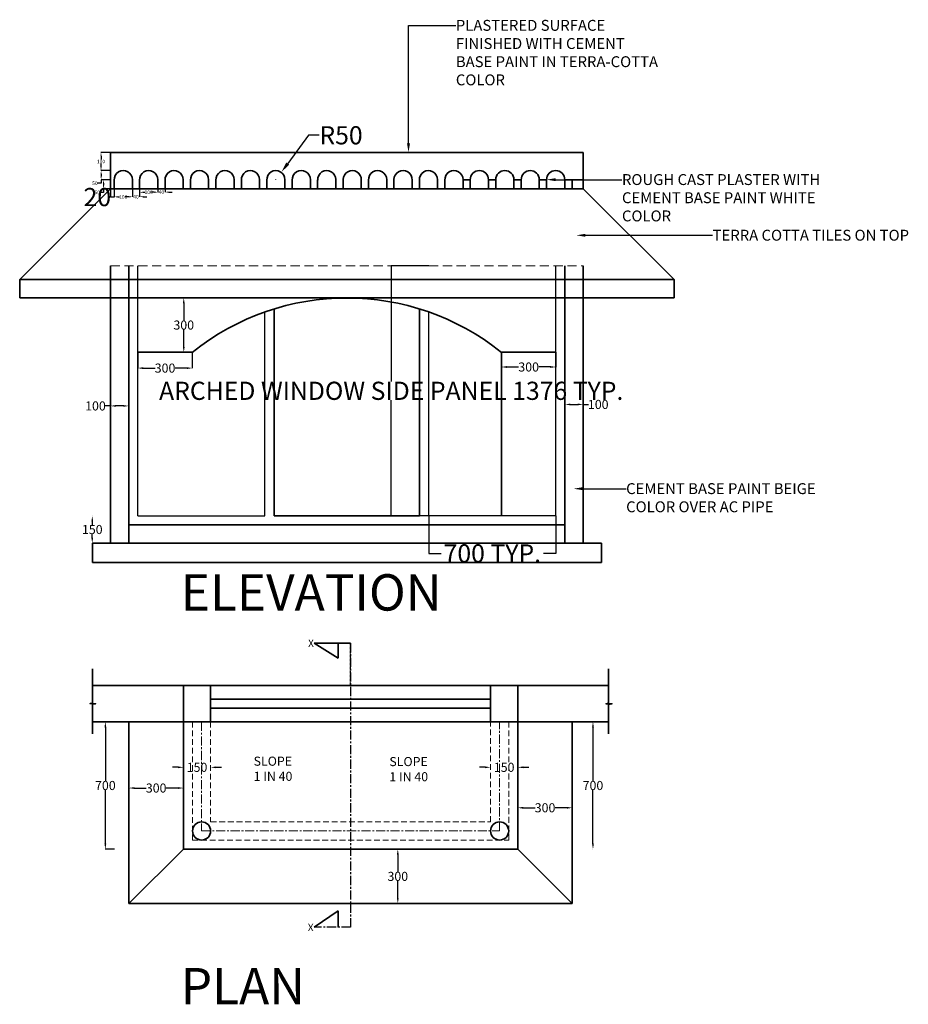
# Model space of a CAD drawing. Units: millimetres. Extents: x 12559 to 31551, y 33148 to 41181.
# Tile 1 of 3: x 12559 to 17450, y 35764 to 41181. Entities that reach past the tile are written whole.
import ezdxf
from ezdxf import colors
from ezdxf.entities.mleader import LeaderData, LeaderLine
from ezdxf.math import Vec2, Vec3

# ---------------------------------------------------------------- set-up
doc = ezdxf.new("R2010")
doc.units = ezdxf.units.MM
doc.header["$MEASUREMENT"] = 0
doc.linetypes.add('CENTER', pattern=[2, 1.25, -0.25, 0.25, -0.25])
doc.linetypes.add('HIDDEN', pattern=[9.525, 6.35, -3.175])
for name, color, linetype, lineweight in [('A-ANNO-DIMS', 2, 'Continuous', 18), ('A-ANNO-SYMB', 2, 'CENTER', 25), ('A-ANNO-TEXT', 3, 'Continuous', 25), ('A-DETL', 7, 'Continuous', 35), ('A-DETL-CNTR', 1, 'CENTER', 18), ('A-DETL-HIDN', 8, 'HIDDEN', 18), ('A-ELEV', 7, 'Continuous', 35), ('A-ELEV-HIDN', 8, 'HIDDEN', 18), ('A-GLAZ', 4, 'Continuous', 25)]:
    doc.layers.add(name, color=color, linetype=linetype, lineweight=lineweight)
doc.styles.get("Standard").update_dxf_attribs({"font": 'arial.ttf'})
doc.dimstyles.get("Standard").update_dxf_attribs({"dimtxt": 100, "dimasz": 0.18, "dimexe": 0.18, "dimexo": 0.0625, "dimgap": 0.09, "dimtad": 0, "dimtih": 1, "dimtoh": 1, "dimdec": 0, "dimzin": 0, "dimdsep": 46, "dimtxsty": 'Standard', "dimcen": 0.09, "dimadec": 0, "dimazin": 0, "dimtfac": 1, "dimtdec": 0, "dimtofl": 0, "dimtmove": 0, "dimatfit": 3, "dimfxl": 1, "dimtolj": 1, "dimtzin": 0, "dimarcsym": 0})

# ---------------------------------------------------------------- blocks, each defined once
blk = doc.blocks.new('*D2')
at = {"layer": 'A-ANNO-DIMS', "color": 0, "lineweight": -2, "transparency": 16777216}
for p, q in [((13430.3, 37067.5), (13400.3, 37067.5)), ((13460.3, 37067.6), (13460.3, 37067.7)), ((13610.3, 37067.6), (13610.3, 37067.7)), ((13640.3, 37067.5), (13670.3, 37067.5))]:
    blk.add_line(p, q, dxfattribs=at)
at = {"layer": 'A-ANNO-DIMS', "color": 0, "transparency": 16777216}
for points in [[(13430.3, 37072.5), (13430.3, 37062.5), (13460.3, 37067.5)], [(13640.3, 37072.5), (13640.3, 37062.5), (13610.3, 37067.5)]]:
    blk.add_solid(points, dxfattribs=at)
at = {"layer": 'DEFPOINTS', "color": 0, "transparency": 16777216}
for p in [(13460.3, 37067.5), (13610.3, 37067.5), (13610.3, 37067.5)]:
    blk.add_point(p, dxfattribs=at)
at = {"layer": 'A-ANNO-DIMS', "color": 0, "transparency": 16777216, "insert": (13535.3, 37067.5), "char_height": 50, "attachment_point": 5}
blk.add_mtext('\\A1;150', dxfattribs=at)
blk = doc.blocks.new('*D3')
at = {"layer": 'A-ANNO-DIMS', "color": 0, "lineweight": -2, "transparency": 16777216}
for p, q in [((15120.7, 37067.5), (15090.7, 37067.5)), ((15150.7, 37067.6), (15150.7, 37067.7)), ((15300.7, 37067.6), (15300.7, 37067.7)), ((15330.7, 37067.5), (15360.7, 37067.5))]:
    blk.add_line(p, q, dxfattribs=at)
at = {"layer": 'A-ANNO-DIMS', "color": 0, "transparency": 16777216}
for points in [[(15120.7, 37072.5), (15120.7, 37062.5), (15150.7, 37067.5)], [(15330.7, 37072.5), (15330.7, 37062.5), (15300.7, 37067.5)]]:
    blk.add_solid(points, dxfattribs=at)
at = {"layer": 'DEFPOINTS', "color": 0, "transparency": 16777216}
for p in [(15150.7, 37067.5), (15300.7, 37067.5), (15300.7, 37067.5)]:
    blk.add_point(p, dxfattribs=at)
at = {"layer": 'A-ANNO-DIMS', "color": 0, "transparency": 16777216, "insert": (15225.7, 37067.5), "char_height": 50, "attachment_point": 5}
blk.add_mtext('\\A1;150', dxfattribs=at)
blk = doc.blocks.new('*D4')
at = {"layer": 'A-ANNO-DIMS', "color": 0, "lineweight": -2, "transparency": 16777216}
for p, q in [((15300.7, 36794.6), (15300.7, 36845.1)), ((15330.7, 36844.9), (15395.5, 36844.9)), ((15570.7, 36844.9), (15505.9, 36844.9)), ((15600.7, 36794.6), (15600.7, 36845.1))]:
    blk.add_line(p, q, dxfattribs=at)
at = {"layer": 'A-ANNO-DIMS', "color": 0, "transparency": 16777216}
for points in [[(15330.7, 36849.9), (15330.7, 36839.9), (15300.7, 36844.9)], [(15570.7, 36849.9), (15570.7, 36839.9), (15600.7, 36844.9)]]:
    blk.add_solid(points, dxfattribs=at)
at = {"layer": 'DEFPOINTS', "color": 0, "transparency": 16777216}
for p in [(15600.7, 36844.9), (15300.7, 36794.6), (15600.7, 36794.6)]:
    blk.add_point(p, dxfattribs=at)
at = {"layer": 'A-ANNO-DIMS', "color": 0, "transparency": 16777216, "insert": (15450.7, 36844.9), "char_height": 50, "attachment_point": 5}
blk.add_mtext('\\A1;300', dxfattribs=at)
blk = doc.blocks.new('*D5')
at = {"layer": 'A-ANNO-DIMS', "color": 0, "lineweight": -2, "transparency": 16777216}
for p, q in [((13160.3, 36897.9), (13160.3, 36953.7)), ((13190.3, 36953.5), (13255.1, 36953.5)), ((13430.3, 36953.5), (13365.5, 36953.5)), ((13460.3, 36897.9), (13460.3, 36953.7))]:
    blk.add_line(p, q, dxfattribs=at)
at = {"layer": 'A-ANNO-DIMS', "color": 0, "transparency": 16777216}
for points in [[(13190.3, 36958.5), (13190.3, 36948.5), (13160.3, 36953.5)], [(13430.3, 36958.5), (13430.3, 36948.5), (13460.3, 36953.5)]]:
    blk.add_solid(points, dxfattribs=at)
at = {"layer": 'DEFPOINTS', "color": 0, "transparency": 16777216}
for p in [(13460.3, 36953.5), (13160.3, 36897.9), (13460.3, 36897.9)]:
    blk.add_point(p, dxfattribs=at)
at = {"layer": 'A-ANNO-DIMS', "color": 0, "transparency": 16777216, "insert": (13310.3, 36953.5), "char_height": 50, "attachment_point": 5}
blk.add_mtext('\\A1;300', dxfattribs=at)
blk = doc.blocks.new('*D6')
at = {"layer": 'A-ANNO-DIMS', "color": 0, "lineweight": -2, "transparency": 16777216}
for p, q in [((13081, 37317.5), (13030.5, 37317.5)), ((13030.7, 37287.5), (13030.7, 36993.1)), ((13030.7, 36647.5), (13030.7, 36941.9)), ((13081, 36617.5), (13030.5, 36617.5))]:
    blk.add_line(p, q, dxfattribs=at)
at = {"layer": 'A-ANNO-DIMS', "color": 0, "transparency": 16777216}
for points in [[(13025.7, 37287.5), (13035.7, 37287.5), (13030.7, 37317.5)], [(13025.7, 36647.5), (13035.7, 36647.5), (13030.7, 36617.5)]]:
    blk.add_solid(points, dxfattribs=at)
at = {"layer": 'DEFPOINTS', "color": 0, "transparency": 16777216}
for p in [(13030.7, 37317.5), (13081.1, 37317.5), (13081.1, 36617.5)]:
    blk.add_point(p, dxfattribs=at)
at = {"layer": 'A-ANNO-DIMS', "color": 0, "transparency": 16777216, "insert": (13030.7, 36967.5), "char_height": 50, "attachment_point": 5}
blk.add_mtext('\\A1;700', dxfattribs=at)
blk = doc.blocks.new('*D7')
at = {"layer": 'A-ANNO-DIMS', "color": 0, "lineweight": -2, "transparency": 16777216}
for p, q in [((15714.4, 37287.5), (15714.4, 36993.1)), ((15714.5, 37317.5), (15714.6, 37317.5)), ((15714.4, 36647.5), (15714.4, 36941.9)), ((15714.5, 36617.5), (15714.6, 36617.5))]:
    blk.add_line(p, q, dxfattribs=at)
at = {"layer": 'A-ANNO-DIMS', "color": 0, "transparency": 16777216}
for points in [[(15709.4, 37287.5), (15719.4, 37287.5), (15714.4, 37317.5)], [(15709.4, 36647.5), (15719.4, 36647.5), (15714.4, 36617.5)]]:
    blk.add_solid(points, dxfattribs=at)
at = {"layer": 'DEFPOINTS', "color": 0, "transparency": 16777216}
for p in [(15714.4, 37317.5), (15714.4, 37317.5), (15714.4, 36617.5)]:
    blk.add_point(p, dxfattribs=at)
at = {"layer": 'A-ANNO-DIMS', "color": 0, "transparency": 16777216, "insert": (15714.4, 36967.5), "char_height": 50, "attachment_point": 5}
blk.add_mtext('\\A1;700', dxfattribs=at)
blk = doc.blocks.new('*D8')
at = {"layer": 'A-ANNO-DIMS', "color": 0, "lineweight": -2, "transparency": 16777216}
for p, q in [((14640.3, 36587.5), (14640.3, 36493.1)), ((14640.4, 36617.5), (14640.5, 36617.5)), ((14640.3, 36347.5), (14640.3, 36441.9)), ((14640.4, 36317.5), (14640.5, 36317.5))]:
    blk.add_line(p, q, dxfattribs=at)
at = {"layer": 'A-ANNO-DIMS', "color": 0, "transparency": 16777216}
for points in [[(14635.3, 36587.5), (14645.3, 36587.5), (14640.3, 36617.5)], [(14635.3, 36347.5), (14645.3, 36347.5), (14640.3, 36317.5)]]:
    blk.add_solid(points, dxfattribs=at)
at = {"layer": 'DEFPOINTS', "color": 0, "transparency": 16777216}
for p in [(14640.3, 36617.5), (14640.3, 36317.5), (14640.3, 36317.5)]:
    blk.add_point(p, dxfattribs=at)
at = {"layer": 'A-ANNO-DIMS', "color": 0, "transparency": 16777216, "insert": (14640.3, 36467.5), "char_height": 50, "attachment_point": 5}
blk.add_mtext('\\A1;300', dxfattribs=at)
blk = doc.blocks.new('*D9')
at = {"layer": 'A-ANNO-DIMS', "color": 0, "lineweight": -2, "transparency": 16777216}
for p, q in [((14148.4, 40545), (14034.3, 40389.5)), ((14208.4, 40545), (14148.4, 40545)), ((13969.1, 40300.8), (13969.3, 40300.8)), ((13969.2, 40300.8), (13969.2, 40300.9))]:
    blk.add_line(p, q, dxfattribs=at)
at = {"layer": 'A-ANNO-DIMS', "color": 0, "transparency": 16777216}
blk.add_solid([(14026.2, 40395.4), (14042.4, 40383.6), (13998.8, 40341.2)], dxfattribs=at)
at = {"layer": 'DEFPOINTS', "color": 0, "transparency": 16777216}
for p in [(13998.8, 40341.2), (13969.2, 40300.8)]:
    blk.add_point(p, dxfattribs=at)
at = {"layer": 'A-ANNO-DIMS', "color": 0, "transparency": 16777216, "insert": (14327.8, 40545), "char_height": 100, "attachment_point": 5}
blk.add_mtext('\\A1;R50', dxfattribs=at)
blk = doc.blocks.new('*D10')
at = {"layer": 'A-ANNO-DIMS', "color": 0, "lineweight": -2, "transparency": 16777216}
for p, q in [((13059.1, 40450.8), (13006.7, 40450.8)), ((13006.8, 40430.8), (13006.8, 40411.2)), ((13006.8, 40370.8), (13006.8, 40390.5)), ((13059.1, 40350.8), (13006.7, 40350.8))]:
    blk.add_line(p, q, dxfattribs=at)
at = {"layer": 'A-ANNO-DIMS', "color": 0, "transparency": 16777216}
for points in [[(13003.5, 40430.8), (13010.2, 40430.8), (13006.8, 40450.8)], [(13003.5, 40370.8), (13010.2, 40370.8), (13006.8, 40350.8)]]:
    blk.add_solid(points, dxfattribs=at)
at = {"layer": 'DEFPOINTS', "color": 0, "transparency": 16777216}
for p in [(13059.2, 40450.8), (13006.8, 40350.8), (13059.2, 40350.8)]:
    blk.add_point(p, dxfattribs=at)
at = {"layer": 'A-ANNO-DIMS', "color": 0, "transparency": 16777216, "insert": (13006.8, 40400.8), "char_height": 20, "attachment_point": 5}
blk.add_mtext('\\A1;100', dxfattribs=at)
blk = doc.blocks.new('*D11')
at = {"layer": 'A-ANNO-DIMS', "color": 0, "lineweight": -2, "transparency": 16777216}
for p, q in [((13059.1, 40350.8), (13007.1, 40350.8)), ((13007.3, 40330.8), (13007.3, 40320.8)), ((13007.3, 40280.8), (12987.3, 40280.8)), ((13059.1, 40300.8), (13007.1, 40300.8)), ((13007.3, 40300.8), (13007.3, 40280.8))]:
    blk.add_line(p, q, dxfattribs=at)
at = {"layer": 'A-ANNO-DIMS', "color": 0, "transparency": 16777216}
for points in [[(13004, 40330.8), (13010.6, 40330.8), (13007.3, 40350.8)], [(13004, 40320.8), (13010.6, 40320.8), (13007.3, 40300.8)]]:
    blk.add_solid(points, dxfattribs=at)
at = {"layer": 'DEFPOINTS', "color": 0, "transparency": 16777216}
for p in [(13059.2, 40350.8), (13007.3, 40300.8), (13059.2, 40300.8)]:
    blk.add_point(p, dxfattribs=at)
at = {"layer": 'A-ANNO-DIMS', "color": 0, "transparency": 16777216, "insert": (12972.9, 40280.8), "char_height": 20, "attachment_point": 5}
blk.add_mtext('\\A1;50', dxfattribs=at)
blk = doc.blocks.new('*D12')
at = {"layer": 'A-ANNO-DIMS', "color": 0, "lineweight": -2, "transparency": 16777216}
for p, q in [((13059.1, 40300.8), (13020.5, 40300.8)), ((13020.7, 40280.8), (13020.7, 40270.8)), ((13020.7, 40230.8), (13000.7, 40230.8)), ((13059.1, 40250.8), (13020.5, 40250.8)), ((13020.7, 40250.8), (13020.7, 40230.8))]:
    blk.add_line(p, q, dxfattribs=at)
at = {"layer": 'A-ANNO-DIMS', "color": 0, "transparency": 16777216}
for points in [[(13017.3, 40280.8), (13024, 40280.8), (13020.7, 40300.8)], [(13017.3, 40270.8), (13024, 40270.8), (13020.7, 40250.8)]]:
    blk.add_solid(points, dxfattribs=at)
at = {"layer": 'DEFPOINTS', "color": 0, "transparency": 16777216}
for p in [(13059.2, 40300.8), (13020.7, 40250.8), (13059.2, 40250.8)]:
    blk.add_point(p, dxfattribs=at)
at = {"layer": 'A-ANNO-DIMS', "color": 0, "transparency": 16777216, "insert": (12986.3, 40230.8), "char_height": 20, "attachment_point": 5}
blk.add_mtext('\\A1;50', dxfattribs=at)
blk = doc.blocks.new('*D13')
at = {"layer": 'A-ANNO-DIMS', "color": 0, "lineweight": -2, "transparency": 16777216}
for p, q in [((13059.2, 40205.1), (13059, 40205.1)), ((13059.2, 40250.8), (13059.2, 40204.9)), ((13079, 40205.1), (13059.4, 40205.1)), ((13079.2, 40250.8), (13079.2, 40204.9))]:
    blk.add_line(p, q, dxfattribs=at)
at = {"layer": 'A-ANNO-DIMS', "color": 0, "transparency": 16777216}
for points in [[(13059.4, 40205.1), (13059.4, 40205), (13059.2, 40205.1)], [(13079, 40205.1), (13079, 40205), (13079.2, 40205.1)]]:
    blk.add_solid(points, dxfattribs=at)
at = {"layer": 'DEFPOINTS', "color": 0, "transparency": 16777216}
for p in [(13059.2, 40250.8), (13059.2, 40205.1), (13079.2, 40250.8)]:
    blk.add_point(p, dxfattribs=at)
at = {"layer": 'A-ANNO-DIMS', "color": 0, "transparency": 16777216, "insert": (12986.6, 40205.1), "char_height": 100, "attachment_point": 5}
blk.add_mtext('\\A1;20', dxfattribs=at)
blk = doc.blocks.new('*D14')
at = {"layer": 'A-ANNO-DIMS', "color": 0, "lineweight": -2, "transparency": 16777216}
for p, q in [((13079.2, 40250.8), (13079.2, 40205.9)), ((13099.2, 40206.1), (13108, 40206.1)), ((13159.2, 40206.1), (13150.4, 40206.1)), ((13179.2, 40250.8), (13179.2, 40205.9))]:
    blk.add_line(p, q, dxfattribs=at)
at = {"layer": 'A-ANNO-DIMS', "color": 0, "transparency": 16777216}
for points in [[(13099.2, 40209.4), (13099.2, 40202.7), (13079.2, 40206.1)], [(13159.2, 40209.4), (13159.2, 40202.7), (13179.2, 40206.1)]]:
    blk.add_solid(points, dxfattribs=at)
at = {"layer": 'DEFPOINTS', "color": 0, "transparency": 16777216}
for p in [(13079.2, 40250.8), (13179.2, 40250.8), (13179.2, 40206.1)]:
    blk.add_point(p, dxfattribs=at)
at = {"layer": 'A-ANNO-DIMS', "color": 0, "transparency": 16777216, "insert": (13129.2, 40206.1), "char_height": 20, "attachment_point": 5}
blk.add_mtext('\\A1;100', dxfattribs=at)
blk = doc.blocks.new('*D15')
at = {"layer": 'A-ANNO-DIMS', "color": 0, "lineweight": -2, "transparency": 16777216}
for p, q in [((13159.2, 40206.9), (13139.2, 40206.9)), ((13179.2, 40250.8), (13179.2, 40206.7)), ((13219.2, 40250.8), (13219.2, 40206.7)), ((13239.2, 40206.9), (13259.2, 40206.9))]:
    blk.add_line(p, q, dxfattribs=at)
at = {"layer": 'A-ANNO-DIMS', "color": 0, "transparency": 16777216}
for points in [[(13159.2, 40210.2), (13159.2, 40203.6), (13179.2, 40206.9)], [(13239.2, 40210.2), (13239.2, 40203.6), (13219.2, 40206.9)]]:
    blk.add_solid(points, dxfattribs=at)
at = {"layer": 'DEFPOINTS', "color": 0, "transparency": 16777216}
for p in [(13179.2, 40250.8), (13219.2, 40250.8), (13219.2, 40206.9)]:
    blk.add_point(p, dxfattribs=at)
at = {"layer": 'A-ANNO-DIMS', "color": 0, "transparency": 16777216, "insert": (13199.2, 40206.9), "char_height": 20, "attachment_point": 5}
blk.add_mtext('\\A1;40', dxfattribs=at)
blk = doc.blocks.new('*D16')
at = {"layer": 'A-ANNO-DIMS', "color": 0, "lineweight": -2, "transparency": 16777216}
for p, q in [((13219.2, 40250.8), (13219.2, 40231.2)), ((13239.2, 40231.4), (13248, 40231.4)), ((13299.2, 40231.4), (13290.4, 40231.4)), ((13319.2, 40250.8), (13319.2, 40231.2))]:
    blk.add_line(p, q, dxfattribs=at)
at = {"layer": 'A-ANNO-DIMS', "color": 0, "transparency": 16777216}
for points in [[(13239.2, 40234.7), (13239.2, 40228.1), (13219.2, 40231.4)], [(13299.2, 40234.7), (13299.2, 40228.1), (13319.2, 40231.4)]]:
    blk.add_solid(points, dxfattribs=at)
at = {"layer": 'DEFPOINTS', "color": 0, "transparency": 16777216}
for p in [(13219.2, 40250.8), (13319.2, 40250.8), (13319.2, 40231.4)]:
    blk.add_point(p, dxfattribs=at)
at = {"layer": 'A-ANNO-DIMS', "color": 0, "transparency": 16777216, "insert": (13269.2, 40231.4), "char_height": 20, "attachment_point": 5}
blk.add_mtext('\\A1;100', dxfattribs=at)
blk = doc.blocks.new('*D17')
at = {"layer": 'A-ANNO-DIMS', "color": 0, "lineweight": -2, "transparency": 16777216}
for p, q in [((13299.2, 40232.4), (13279.2, 40232.4)), ((13319.2, 40250.8), (13319.2, 40232.2)), ((13359.2, 40250.8), (13359.2, 40232.2)), ((13379.2, 40232.4), (13399.2, 40232.4))]:
    blk.add_line(p, q, dxfattribs=at)
at = {"layer": 'A-ANNO-DIMS', "color": 0, "transparency": 16777216}
for points in [[(13299.2, 40235.7), (13299.2, 40229.1), (13319.2, 40232.4)], [(13379.2, 40235.7), (13379.2, 40229.1), (13359.2, 40232.4)]]:
    blk.add_solid(points, dxfattribs=at)
at = {"layer": 'DEFPOINTS', "color": 0, "transparency": 16777216}
for p in [(13319.2, 40250.8), (13359.2, 40250.8), (13359.2, 40232.4)]:
    blk.add_point(p, dxfattribs=at)
at = {"layer": 'A-ANNO-DIMS', "color": 0, "transparency": 16777216, "insert": (13339.2, 40232.4), "char_height": 20, "attachment_point": 5}
blk.add_mtext('\\A1;40', dxfattribs=at)
blk = doc.blocks.new('*D18')
at = {"layer": 'A-ANNO-DIMS', "color": 0, "lineweight": -2, "transparency": 16777216}
for p, q in [((13209.2, 39350.8), (13209.2, 39263.8)), ((13509.2, 39350.8), (13509.2, 39263.8)), ((13239.2, 39264), (13304, 39264)), ((13479.2, 39264), (13414.4, 39264))]:
    blk.add_line(p, q, dxfattribs=at)
at = {"layer": 'A-ANNO-DIMS', "color": 0, "transparency": 16777216}
for points in [[(13239.2, 39269), (13239.2, 39259), (13209.2, 39264)], [(13479.2, 39269), (13479.2, 39259), (13509.2, 39264)]]:
    blk.add_solid(points, dxfattribs=at)
at = {"layer": 'DEFPOINTS', "color": 0, "transparency": 16777216}
for p in [(13209.2, 39350.8), (13509.2, 39350.8), (13209.2, 39264)]:
    blk.add_point(p, dxfattribs=at)
at = {"layer": 'A-ANNO-DIMS', "color": 0, "transparency": 16777216, "insert": (13359.2, 39264), "char_height": 50, "attachment_point": 5}
blk.add_mtext('\\A1;300', dxfattribs=at)
blk = doc.blocks.new('*D19')
at = {"layer": 'A-ANNO-DIMS', "color": 0, "lineweight": -2, "transparency": 16777216}
for p, q in [((13509.1, 39650.8), (13462, 39650.8)), ((13462.2, 39620.8), (13462.2, 39526.5)), ((13462.2, 39380.8), (13462.2, 39475.2)), ((13509.1, 39350.8), (13462, 39350.8))]:
    blk.add_line(p, q, dxfattribs=at)
at = {"layer": 'A-ANNO-DIMS', "color": 0, "transparency": 16777216}
for points in [[(13457.2, 39620.8), (13467.2, 39620.8), (13462.2, 39650.8)], [(13457.2, 39380.8), (13467.2, 39380.8), (13462.2, 39350.8)]]:
    blk.add_solid(points, dxfattribs=at)
at = {"layer": 'DEFPOINTS', "color": 0, "transparency": 16777216}
for p in [(13462.2, 39650.8), (13509.2, 39650.8), (13509.2, 39350.8)]:
    blk.add_point(p, dxfattribs=at)
at = {"layer": 'A-ANNO-DIMS', "color": 0, "transparency": 16777216, "insert": (13462.2, 39500.8), "char_height": 50, "attachment_point": 5}
blk.add_mtext('\\A1;300', dxfattribs=at)
blk = doc.blocks.new('*D20')
at = {"layer": 'A-ANNO-DIMS', "color": 0, "lineweight": -2, "transparency": 16777216}
for p, q in [((15210.5, 39350.8), (15210.5, 39269.9)), ((15510.5, 39350.8), (15510.5, 39269.9)), ((15240.5, 39270.1), (15305.3, 39270.1)), ((15480.5, 39270.1), (15415.7, 39270.1))]:
    blk.add_line(p, q, dxfattribs=at)
at = {"layer": 'A-ANNO-DIMS', "color": 0, "transparency": 16777216}
for points in [[(15240.5, 39275.1), (15240.5, 39265.1), (15210.5, 39270.1)], [(15480.5, 39275.1), (15480.5, 39265.1), (15510.5, 39270.1)]]:
    blk.add_solid(points, dxfattribs=at)
at = {"layer": 'DEFPOINTS', "color": 0, "transparency": 16777216}
for p in [(15210.5, 39350.8), (15510.5, 39350.8), (15510.5, 39270.1)]:
    blk.add_point(p, dxfattribs=at)
at = {"layer": 'A-ANNO-DIMS', "color": 0, "transparency": 16777216, "insert": (15360.5, 39270.1), "char_height": 50, "attachment_point": 5}
blk.add_mtext('\\A1;300', dxfattribs=at)
blk = doc.blocks.new('*D21')
at = {"layer": 'A-ANNO-DIMS', "color": 0, "lineweight": -2, "transparency": 16777216}
for p, q in [((15560.5, 39064.1), (15560.5, 39064.2)), ((15590.5, 39064.1), (15630.5, 39064.1)), ((15660.5, 39064.1), (15660.5, 39064.2)), ((15660.5, 39064.1), (15690.5, 39064.1))]:
    blk.add_line(p, q, dxfattribs=at)
at = {"layer": 'A-ANNO-DIMS', "color": 0, "transparency": 16777216}
for points in [[(15590.5, 39069.1), (15590.5, 39059.1), (15560.5, 39064.1)], [(15630.5, 39069.1), (15630.5, 39059.1), (15660.5, 39064.1)]]:
    blk.add_solid(points, dxfattribs=at)
at = {"layer": 'DEFPOINTS', "color": 0, "transparency": 16777216}
for p in [(15560.5, 39064.1), (15660.5, 39064.1), (15660.5, 39064.1)]:
    blk.add_point(p, dxfattribs=at)
at = {"layer": 'A-ANNO-DIMS', "color": 0, "transparency": 16777216, "insert": (15743.4, 39064.1), "char_height": 50, "attachment_point": 5}
blk.add_mtext('\\A1;100', dxfattribs=at)
blk = doc.blocks.new('*D22')
at = {"layer": 'A-ANNO-DIMS', "color": 0, "lineweight": -2, "transparency": 16777216}
for p, q in [((13059.2, 39064), (13059.2, 39055.7)), ((13159.2, 39064), (13159.2, 39055.7)), ((13059.2, 39055.9), (13029.2, 39055.9)), ((13129.2, 39055.9), (13089.2, 39055.9))]:
    blk.add_line(p, q, dxfattribs=at)
at = {"layer": 'A-ANNO-DIMS', "color": 0, "transparency": 16777216}
for points in [[(13089.2, 39060.9), (13089.2, 39050.9), (13059.2, 39055.9)], [(13129.2, 39060.9), (13129.2, 39050.9), (13159.2, 39055.9)]]:
    blk.add_solid(points, dxfattribs=at)
at = {"layer": 'DEFPOINTS', "color": 0, "transparency": 16777216}
for p in [(13059.2, 39064.1), (13159.2, 39064.1), (13059.2, 39055.9)]:
    blk.add_point(p, dxfattribs=at)
at = {"layer": 'A-ANNO-DIMS', "color": 0, "transparency": 16777216, "insert": (12976.3, 39055.9), "char_height": 50, "attachment_point": 5}
blk.add_mtext('\\A1;100', dxfattribs=at)
blk = doc.blocks.new('*D23')
at = {"layer": 'A-ANNO-DIMS', "color": 0, "lineweight": -2, "transparency": 16777216}
for p, q in [((12958.7, 38420.8), (12958.7, 38401.5)), ((12958.8, 38450.8), (12958.9, 38450.8)), ((12958.7, 38330.8), (12958.7, 38350.2)), ((12958.8, 38300.8), (12958.9, 38300.8))]:
    blk.add_line(p, q, dxfattribs=at)
at = {"layer": 'A-ANNO-DIMS', "color": 0, "transparency": 16777216}
for points in [[(12953.7, 38420.8), (12963.7, 38420.8), (12958.7, 38450.8)], [(12953.7, 38330.8), (12963.7, 38330.8), (12958.7, 38300.8)]]:
    blk.add_solid(points, dxfattribs=at)
at = {"layer": 'DEFPOINTS', "color": 0, "transparency": 16777216}
for p in [(12958.7, 38450.8), (12958.7, 38300.8), (12958.7, 38300.8)]:
    blk.add_point(p, dxfattribs=at)
at = {"layer": 'A-ANNO-DIMS', "color": 0, "transparency": 16777216, "insert": (12958.7, 38375.8), "char_height": 50, "attachment_point": 5}
blk.add_mtext('\\A1;150', dxfattribs=at)
blk = doc.blocks.new('TERRACOTTA-TILE')
for p, q in [((0, 0), (0, 50)), ((100, 0), (100, 50))]:
    blk.add_line(p, q)
blk.add_arc((50, 50), 50, 0, 182.662)
blk = doc.blocks.new('TERRACOTTA-TILE-END')
for p, q in [((0, 0), (0, 50)), ((0, 0), (0, 50)), ((100, 0), (100, 50))]:
    blk.add_line(p, q)
blk.add_arc((50, 50), 50, 0, 182.662)
blk = doc.blocks.new('WIN-ARCH-SIDE')
for points in [[(0, 0), (0, 1376.4)], [(700, 0), (700, 1122.1)], [(0, 0), (700, 0)]]:
    blk.add_lwpolyline(points)
blk = doc.blocks.new('*D38')
at = {"layer": 'A-ANNO-DIMS', "color": 0, "lineweight": -2, "transparency": 16777216}
for p, q in [((14810.4, 39827.3), (14603.9, 39827.3)), ((14604, 39827.1), (14604, 39190.9)), ((14604, 38451), (14604, 39087.2)), ((14810.4, 38450.8), (14603.9, 38450.8))]:
    blk.add_line(p, q, dxfattribs=at)
at = {"layer": 'A-ANNO-DIMS', "color": 0, "transparency": 16777216}
for points in [[(14604, 39827.1), (14604.1, 39827.1), (14604, 39827.3)], [(14604, 38451), (14604.1, 38451), (14604, 38450.8)]]:
    blk.add_solid(points, dxfattribs=at)
at = {"layer": 'DEFPOINTS', "color": 0, "transparency": 16777216}
for p in [(14604, 39827.3), (14810.5, 39827.3), (14810.5, 38450.8)]:
    blk.add_point(p, dxfattribs=at)
at = {"layer": 'A-ANNO-DIMS', "color": 0, "transparency": 16777216, "insert": (14604, 39139.1), "char_height": 100, "attachment_point": 5}
blk.add_mtext('\\A1;ARCHED WINDOW SIDE PANEL 1376 TYP.', dxfattribs=at)
blk = doc.blocks.new('*D39')
at = {"layer": 'A-ANNO-DIMS', "color": 0, "lineweight": -2, "transparency": 16777216}
for p, q in [((14810.5, 38450.8), (14810.5, 38244.2)), ((15510.5, 38450.8), (15510.5, 38244.2)), ((14810.7, 38244.4), (14878.6, 38244.4)), ((15510.3, 38244.4), (15442.4, 38244.4))]:
    blk.add_line(p, q, dxfattribs=at)
at = {"layer": 'A-ANNO-DIMS', "color": 0, "transparency": 16777216}
for points in [[(14810.7, 38244.4), (14810.7, 38244.4), (14810.5, 38244.4)], [(15510.3, 38244.4), (15510.3, 38244.4), (15510.5, 38244.4)]]:
    blk.add_solid(points, dxfattribs=at)
at = {"layer": 'DEFPOINTS', "color": 0, "transparency": 16777216}
for p in [(14810.5, 38450.8), (15510.5, 38450.8), (14810.5, 38244.4)]:
    blk.add_point(p, dxfattribs=at)
at = {"layer": 'A-ANNO-DIMS', "color": 0, "transparency": 16777216, "insert": (15160.5, 38244.4), "char_height": 100, "attachment_point": 5}
blk.add_mtext('\\A1;700 TYP.', dxfattribs=at)

msp = doc.modelspace()

# ---------------------------------------------------------------- linework, layer by layer
at = {"layer": 'A-ANNO-SYMB'}
msp.add_line((14380.5, 37517.5), (14380.5, 37749.8), dxfattribs=at)
at = {"layer": 'A-ANNO-SYMB', "ltscale": 40}
for p, q in [((14380.5, 37749.8), (14380.5, 36317.5)), ((14380.5, 36317.5), (14380.5, 36188.2)), ((14380.5, 36188.2), (14180.5, 36188.2))]:
    msp.add_line(p, q, dxfattribs=at)
at = {"layer": 'A-DETL'}
for p, q in [((14380.5, 37749.8), (14180.5, 37749.8)), ((14180.5, 37749.8), (14312.4, 37667.3)), ((14312.4, 37667.3), (14312.4, 37749.8)), ((12960.3, 37517.5), (12960.3, 37608.5)), ((15800.7, 37517.5), (15800.7, 37608.5)), ((15800.7, 37517.5), (12960.3, 37517.5)), ((12960.3, 37317.5), (12960.3, 37517.5)), ((13460.3, 37517.5), (13460.3, 36617.5)), ((13610.3, 37317.5), (13610.3, 37517.5)), ((15150.7, 37317.5), (15150.7, 37517.5)), ((15300.7, 36617.5), (15300.7, 37517.5)), ((15800.7, 37420.8), (15800.7, 37517.5)), ((13610.3, 37442.5), (15150.7, 37442.5)), ((13610.3, 37392.5), (15150.7, 37392.5)), ((15800.7, 37317.5), (15800.7, 37413)), ((15800.7, 37317.5), (12960.3, 37317.5)), ((12960.3, 37317.5), (12960.3, 37251.5)), ((13160.3, 37317.5), (13160.3, 36317.5)), ((15600.7, 36617.5), (15600.7, 37317.5)), ((15800.7, 37251.5), (15800.7, 37317.5)), ((13460.3, 36617.5), (13160.3, 36317.5)), ((13460.3, 36617.5), (15300.7, 36617.5)), ((15300.7, 36617.5), (15600.7, 36317.5)), ((15600.7, 36617.5), (15600.7, 36317.5)), ((13160.3, 36317.5), (15600.7, 36317.5)), ((14180.5, 36188.2), (14312.4, 36278.1)), ((14312.4, 36278.1), (14312.4, 36188.2))]:
    msp.add_line(p, q, dxfattribs=at)
for points in [[(12960.3, 37517.7), (12960.3, 37419.8), (12946.5, 37418.5), (12977.2, 37417.3), (12960.3, 37414.9), (12960.3, 37317.3)], [(15800.7, 37317.3), (15800.7, 37413), (15819.5, 37417.4), (15785.3, 37417.6), (15800.7, 37420.8), (15800.7, 37517.7)]]:
    msp.add_lwpolyline(points, dxfattribs=at)
for centre in [(13560.3, 36717.5), (15200.7, 36717.5)]:
    msp.add_circle(centre, 50, dxfattribs=at)
at = {"layer": 'A-DETL-CNTR', "ltscale": 40}
for p, q in [((13560.3, 37317.5), (13560.3, 36717.5)), ((15200.7, 36717.5), (15200.7, 37317.5)), ((13560.3, 36717.5), (15200.7, 36717.5))]:
    msp.add_line(p, q, dxfattribs=at)
at = {"layer": 'A-DETL-HIDN', "ltscale": 5}
for p, q in [((13510.3, 37317.5), (13510.3, 36667.5)), ((13610.3, 37317.5), (13610.3, 36767.5)), ((15150.7, 36767.5), (15150.7, 37317.5)), ((15250.7, 36667.5), (15250.7, 37317.5)), ((13610.3, 36767.5), (15150.7, 36767.5)), ((13510.3, 36667.5), (15250.7, 36667.5))]:
    msp.add_line(p, q, dxfattribs=at)
at = {"layer": 'A-ELEV'}
for p, q in [((13059.2, 40250.8), (13059.2, 40450.8)), ((15660.5, 40450.8), (15660.5, 40250.8)), ((14759.2, 40250.8), (14759.2, 40300.8)), ((14759.2, 40250.8), (14759.2, 40300.8)), ((14759.2, 40250.8), (14759.2, 40300.8)), ((14859.2, 40250.8), (14859.2, 40300.8)), ((14899.2, 40250.8), (14899.2, 40300.8)), ((14999.2, 40250.8), (14999.2, 40300.8)), ((14999.2, 40250.8), (14999.2, 40300.8)), ((15039.2, 40250.8), (15039.2, 40300.8)), ((15039.2, 40250.8), (15039.2, 40300.8)), ((15039.2, 40250.8), (15039.2, 40300.8)), ((15139.2, 40250.8), (15139.2, 40300.8)), ((15179.2, 40250.8), (15179.2, 40300.8)), ((15279.2, 40250.8), (15279.2, 40300.8)), ((15279.2, 40250.8), (15279.2, 40300.8)), ((15319.2, 40250.8), (15319.2, 40300.8)), ((15319.2, 40250.8), (15319.2, 40300.8)), ((15319.2, 40250.8), (15319.2, 40300.8)), ((15419.2, 40250.8), (15419.2, 40300.8)), ((15459.2, 40250.8), (15459.2, 40300.8)), ((15559.2, 40250.8), (15559.2, 40300.8)), ((15599.2, 40250.8), (15599.2, 40300.8)), ((12559.2, 39750.8), (13059.2, 40250.8)), ((16160.5, 39750.8), (15660.5, 40250.8))]:
    msp.add_line(p, q, dxfattribs=at)
for points in [[(13059.2, 40450.8), (15660.5, 40450.8)], [(14999.2, 40300.8), (15039.2, 40300.8)], [(15139.2, 40300.8), (15179.2, 40300.8)], [(15279.2, 40300.8), (15319.2, 40300.8)], [(15419.2, 40300.8), (15459.2, 40300.8)], [(15559.2, 40300.8), (15660.5, 40300.8)], [(13059.2, 40250.8), (15660.5, 40250.8)], [(13059.2, 38300.8), (13059.2, 39827.3)], [(13159.2, 38300.8), (13159.2, 39827.3)], [(15560.5, 39827.3), (15560.5, 38300.8)], [(15660.5, 39827.3), (15660.5, 38300.8)], [(12559.2, 39650.8), (12559.2, 39750.8)], [(12559.2, 39750.8), (16160.5, 39750.8)], [(16160.5, 39750.8), (16160.5, 39650.8)], [(12559.2, 39650.8), (16160.5, 39650.8)], [(13959.2, 38450.8), (13959.2, 39589.4)], [(14760.5, 39589.4), (14760.5, 38450.8)], [(13209.2, 39350.8), (13509.2, 39350.8)], [(15210.5, 39350.8), (15210.5, 38450.8)], [(15210.5, 39350.8), (15510.5, 39350.8)], [(13959.2, 38450.8), (14760.5, 38450.8)], [(13159.2, 38400.8), (15560.5, 38400.8)], [(12959.2, 38300.8), (15760.5, 38300.8)], [(12959.2, 38195.1), (12959.2, 38300.8)], [(15760.5, 38300.8), (15760.5, 38195.1)], [(15760.5, 38195.1), (12959.2, 38195.1)]]:
    msp.add_lwpolyline(points, dxfattribs=at)
for centre, radius, start, end in [((14809.2, 40300.8), 50, 0, 182.662), ((14949.2, 40300.8), 50, 0, 182.662), ((15089.2, 40300.8), 50, 0, 180), ((15229.2, 40300.8), 50, 0, 180), ((15369.2, 40300.8), 50, 0, 180), ((15509.2, 40300.8), 50, 0, 180), ((14359.9, 38290), 1359.7, 51.2742, 128.7258)]:
    msp.add_arc(centre, radius, start, end, dxfattribs=at)
at = {"layer": 'A-ELEV-HIDN', "ltscale": 8}
msp.add_line((13059.2, 39827.3), (15660.5, 39827.3), dxfattribs=at)

# ---------------------------------------------------------------- block references
at = {"layer": 'A-ELEV'}
for name, p in [('TERRACOTTA-TILE', (13079.2, 40250.8)), ('TERRACOTTA-TILE', (13219.2, 40250.8)), ('TERRACOTTA-TILE-END', (13359.2, 40250.8)), ('TERRACOTTA-TILE', (13499.2, 40250.8)), ('TERRACOTTA-TILE', (13639.2, 40250.8)), ('TERRACOTTA-TILE', (13779.2, 40250.8)), ('TERRACOTTA-TILE-END', (13919.2, 40250.8)), ('TERRACOTTA-TILE', (14059.2, 40250.8))]:
    msp.add_blockref(name, p, dxfattribs=at)
for name, p, rotation in [('TERRACOTTA-TILE', (14199.2, 40250.8), 0.012495283461489), ('TERRACOTTA-TILE-END', (14479.2, 40250.8), 0.0070579219566126)]:
    msp.add_blockref(name, p, dxfattribs=dict(at, rotation=rotation))
at = {"layer": 'A-ELEV', "extrusion": (0, 0, -1), "zscale": -1, "rotation": 359.997646645306}
for p in [(-14439.2, 40250.9), (-14719.2, 40250.9)]:
    msp.add_blockref('TERRACOTTA-TILE-END', p, dxfattribs=at)
at = {"layer": 'A-GLAZ'}
msp.add_blockref('WIN-ARCH-SIDE', (13209.2, 38450.8), dxfattribs=at)
at = {"layer": 'A-GLAZ', "extrusion": (0, 0, -1), "zscale": -1}
msp.add_blockref('WIN-ARCH-SIDE', (-15510.5, 38450.8), dxfattribs=at)

# ---------------------------------------------------------------- texts
at = {"layer": 'A-ANNO-TEXT', "attachment_point": 1}
for s, width, insert, char_height in [('ELEVATION', 1537.626, (13445.8, 38129.9), 200), ('X', 163.128, (14146.8, 37769.8), 40), ('{\\H250x;SLOPE\\P1 IN 40}', 1051.995, (13846.6, 37126.3), 0.2), ('{\\H250x;SLOPE\\P1 IN 40}', 1051.995, (14593.7, 37124.1), 0.2), ('X', 163.128, (14145, 36206.4), 40), ('PLAN', 1537.626, (13445.8, 35963.5), 200)]:
    msp.add_mtext_dynamic_manual_height_columns(s, width=width, gutter_width=1, heights=[0], dxfattribs=dict(at, insert=insert, char_height=char_height))

# ---------------------------------------------------------------- dimensions: what is measured, and where the dimension line sits
at = {"layer": 'A-ANNO-DIMS'}
dim = msp.add_radius_dim(center=(13969.2, 40300.8), mpoint=(13998.8, 40341.2), dimstyle='Standard', override={"dimasz": 60, "dimclrd": 0, "dimclre": 0, "dimclrt": 0}, dxfattribs=at)
dim.commit()
dim.dimension.update_dxf_attribs({"geometry": '*D9', "text_midpoint": (14327.8, 40545), "dimtype": 164})
for base, p1, p2, override, picture, middle in [((13006.8, 40350.8), (13059.2, 40450.8), (13059.2, 40350.8), {"dimtxt": 20, "dimasz": 20, "dimclrd": 0, "dimclre": 0, "dimclrt": 0}, '*D10', (13006.8, 40400.8)), ((13007.3, 40300.8), (13059.2, 40350.8), (13059.2, 40300.8), {"dimtxt": 20, "dimasz": 20, "dimclrd": 0, "dimclre": 0, "dimclrt": 0}, '*D11', (12972.9, 40280.8)), ((13020.7, 40250.8), (13059.2, 40300.8), (13059.2, 40250.8), {"dimtxt": 20, "dimasz": 20, "dimclrd": 0, "dimclre": 0, "dimclrt": 0}, '*D12', (12986.3, 40230.8)), ((13462.2, 39650.8), (13509.2, 39350.8), (13509.2, 39650.8), {"dimtxt": 50, "dimasz": 30, "dimclrd": 0, "dimclre": 0, "dimclrt": 0}, '*D19', (13462.2, 39500.8)), ((12958.7, 38300.8), (12958.7, 38450.8), (12958.7, 38300.8), {"dimtxt": 50, "dimasz": 30, "dimclrd": 0, "dimclre": 0, "dimclrt": 0}, '*D23', (12958.7, 38375.8)), ((13030.7, 37317.5), (13081.1, 36617.5), (13081.1, 37317.5), {"dimtxt": 50, "dimasz": 30, "dimclrd": 0, "dimclre": 0, "dimclrt": 0}, '*D6', (13030.7, 36967.5)), ((15714.4, 37317.5), (15714.4, 36617.5), (15714.4, 37317.5), {"dimtxt": 50, "dimasz": 30, "dimclrd": 0, "dimclre": 0, "dimclrt": 0}, '*D7', (15714.4, 36967.5)), ((14640.3, 36317.5), (14640.3, 36617.5), (14640.3, 36317.5), {"dimtxt": 50, "dimasz": 30, "dimclrd": 0, "dimclre": 0, "dimclrt": 0}, '*D8', (14640.3, 36467.5))]:
    dim = msp.add_linear_dim(base=base, p1=p1, p2=p2, angle=90, dimstyle='Standard', override=override, dxfattribs=at)
    dim.commit()
    dim.dimension.update_dxf_attribs({"geometry": picture, "text_midpoint": middle})
for base, p1, p2, override, picture, middle in [((13059.2, 40205.1), (13079.2, 40250.8), (13059.2, 40250.8), {"dimclrd": 0, "dimclre": 0, "dimclrt": 0}, '*D13', (12986.6, 40205.1)), ((13179.2, 40206.1), (13079.2, 40250.8), (13179.2, 40250.8), {"dimtxt": 20, "dimasz": 20, "dimclrd": 0, "dimclre": 0, "dimclrt": 0}, '*D14', (13129.2, 40206.1)), ((13219.2, 40206.9), (13179.2, 40250.8), (13219.2, 40250.8), {"dimtxt": 20, "dimasz": 20, "dimclrd": 0, "dimclre": 0, "dimclrt": 0}, '*D15', (13199.2, 40206.9)), ((13319.2, 40231.4), (13219.2, 40250.8), (13319.2, 40250.8), {"dimtxt": 20, "dimasz": 20, "dimclrd": 0, "dimclre": 0, "dimclrt": 0}, '*D16', (13269.2, 40231.4)), ((13359.2, 40232.4), (13319.2, 40250.8), (13359.2, 40250.8), {"dimtxt": 20, "dimasz": 20, "dimclrd": 0, "dimclre": 0, "dimclrt": 0}, '*D17', (13339.2, 40232.4)), ((13209.2, 39264), (13509.2, 39350.8), (13209.2, 39350.8), {"dimtxt": 50, "dimasz": 30, "dimclrd": 0, "dimclre": 0, "dimclrt": 0}, '*D18', (13359.2, 39264)), ((15510.5, 39270.1), (15210.5, 39350.8), (15510.5, 39350.8), {"dimtxt": 50, "dimasz": 30, "dimclrd": 0, "dimclre": 0, "dimclrt": 0}, '*D20', (15360.5, 39270.1)), ((13059.2, 39055.9), (13159.2, 39064.1), (13059.2, 39064.1), {"dimtxt": 50, "dimasz": 30, "dimclrd": 0, "dimclre": 0, "dimclrt": 0}, '*D22', (12976.3, 39055.9)), ((15660.5, 39064.1), (15560.5, 39064.1), (15660.5, 39064.1), {"dimtxt": 50, "dimasz": 30, "dimclrd": 0, "dimclre": 0, "dimclrt": 0}, '*D21', (15743.4, 39064.1)), ((13610.3, 37067.5), (13460.3, 37067.5), (13610.3, 37067.5), {"dimtxt": 50, "dimasz": 30, "dimclrd": 0, "dimclre": 0, "dimclrt": 0}, '*D2', (13535.3, 37067.5)), ((15300.7, 37067.5), (15150.7, 37067.5), (15300.7, 37067.5), {"dimtxt": 50, "dimasz": 30, "dimclrd": 0, "dimclre": 0, "dimclrt": 0}, '*D3', (15225.7, 37067.5)), ((13460.3, 36953.5), (13160.3, 36897.9), (13460.3, 36897.9), {"dimtxt": 50, "dimasz": 30, "dimclrd": 0, "dimclre": 0, "dimclrt": 0}, '*D5', (13310.3, 36953.5)), ((15600.7, 36844.9), (15300.7, 36794.6), (15600.7, 36794.6), {"dimtxt": 50, "dimasz": 30, "dimclrd": 0, "dimclre": 0, "dimclrt": 0}, '*D4', (15450.7, 36844.9))]:
    dim = msp.add_linear_dim(base=base, p1=p1, p2=p2, dimstyle='Standard', override=override, dxfattribs=at)
    dim.commit()
    dim.dimension.update_dxf_attribs({"geometry": picture, "text_midpoint": middle})
for base, p1, p2, angle, text, picture, middle in [((14604.0411, 39827.2574), (14810.5022, 38450.8495), (14810.5022, 39827.2574), 90, 'ARCHED WINDOW SIDE PANEL <> TYP.', '*D38', (14604.0411, 39139.0535)), ((14810.5, 38244.4), (15510.5, 38450.8), (14810.5, 38450.8), 180, '<> TYP.', '*D39', (15160.5, 38244.4))]:
    dim = msp.add_linear_dim(base=base, p1=p1, p2=p2, angle=angle, text=text, dimstyle='Standard', override={"dimdec": 0, "dimrnd": 0, "dimzin": 0, "dimlunit": 2}, dxfattribs=at)
    dim.commit()
    dim.dimension.update_dxf_attribs({"geometry": picture, "text_midpoint": middle})

# ---------------------------------------------------------------- leaders
at = {"layer": 'A-ANNO-TEXT'}
ml = msp.add_multileader_mtext('Standard', dxfattribs=at)
ml.set_content('PLASTERED SURFACE \\PFINISHED WITH CEMENT\\PBASE PAINT IN TERRA-COTTA\\PCOLOR', color=256)
ml.set_leader_properties()
ml.build(insert=Vec2(0, 0))
ml.multileader.update_dxf_attribs({"dogleg_length": 0.36, "arrow_head_size": 50})
ctx = ml.context
ctx.base_point, ctx.char_height, ctx.arrow_head_size, ctx.landing_gap_size, ctx.plane_origin = Vec3(14959.7, 41149.4), 60, 50, 0.09, Vec3(14699.2, 40450.8)
notes = []
notes.append((ctx, [(0, (1, 1, 0), (14699.2, 41149.4), (1, 0), 260.5, [(0, [(14699.2, 40450.8)], 0, [])])]))
ctx.mtext.insert, ctx.mtext.flow_direction = Vec3(14959.8, 41179.9), 5
ml = msp.add_multileader_mtext('Standard', dxfattribs=at)
ml.set_content('ROUGH CAST PLASTER WITH \\PCEMENT BASE PAINT WHITE\\PCOLOR', color=256)
ml.set_leader_properties()
ml.build(insert=Vec2(0, 0))
ml.multileader.update_dxf_attribs({"dogleg_length": 0.36, "arrow_head_size": 50})
ctx = ml.context
ctx.base_point, ctx.char_height, ctx.arrow_head_size, ctx.landing_gap_size, ctx.plane_origin = Vec3(15874, 40300.8), 60, 50, 0.09, Vec3(15459.2, 40300.8)
notes.append((ctx, [(0, (1, 1, 0), (15873.7, 40300.8), (1, 0), 0.36, [(0, [(15459.2, 40300.8)], 0, [])])]))
ctx.mtext.insert, ctx.mtext.flow_direction = Vec3(15874.1, 40331.4), 5
ml = msp.add_multileader_mtext('Standard', dxfattribs=at)
ml.set_content('TERRA COTTA TILES ON TOP', color=256)
ml.set_leader_properties()
ml.build(insert=Vec2(0, 0))
ml.multileader.update_dxf_attribs({"dogleg_length": 0.36, "arrow_head_size": 50})
ctx = ml.context
ctx.base_point, ctx.char_height, ctx.arrow_head_size, ctx.landing_gap_size, ctx.plane_origin = Vec3(16372.9, 39994.7), 60, 50, 0.09, Vec3(15622.8, 39994.7)
notes.append((ctx, [(0, (1, 1, 0), (16372.5, 39994.7), (1, 0), 0.36, [(0, [(15622.8, 39994.7)], 0, [])])]))
ctx.mtext.insert, ctx.mtext.flow_direction = Vec3(16373, 40025.2), 5
ml = msp.add_multileader_mtext('Standard', dxfattribs=at)
ml.set_content('CEMENT BASE PAINT BEIGE\\PCOLOR OVER AC PIPE', color=256)
ml.set_leader_properties()
ml.build(insert=Vec2(0, 0))
ml.multileader.update_dxf_attribs({"dogleg_length": 0.36, "arrow_head_size": 50})
ctx = ml.context
ctx.base_point, ctx.char_height, ctx.arrow_head_size, ctx.landing_gap_size, ctx.plane_origin = Vec3(15896.8, 38600.4), 60, 50, 0.09, Vec3(15608.6, 38600.4)
notes.append((ctx, [(0, (1, 1, 0), (15896.4, 38600.4), (1, 0), 0.36, [(0, [(15608.6, 38600.4)], 0, [])])]))
ctx.mtext.insert, ctx.mtext.flow_direction = Vec3(15896.9, 38630.9), 5
for ctx, leaders in notes:
    for number, flags, end, landing, length, lines in leaders:
        leader = LeaderData()
        leader.index, (leader.has_last_leader_line, leader.has_dogleg_vector, leader.attachment_direction) = number, flags
        leader.last_leader_point, leader.dogleg_vector, leader.dogleg_length = Vec3(end), Vec3(landing), length
        for number, points, colour, breaks in lines:
            line = LeaderLine()
            line.index, line.vertices, line.color, line.breaks = number, Vec3.list(points), colors.encode_raw_color(colour), breaks
            leader.lines.append(line)
        ctx.leaders.append(leader)

doc.saveas('drawing.dxf')
